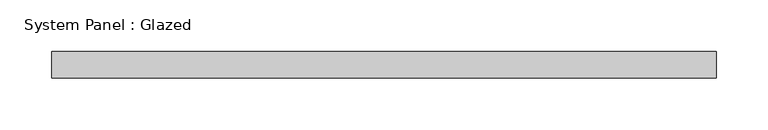
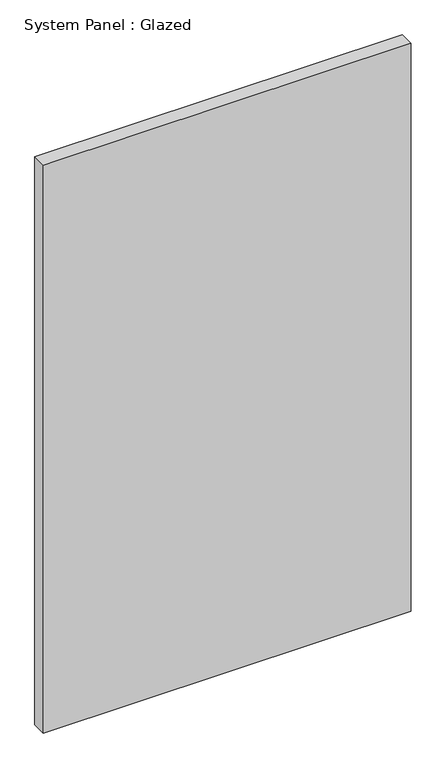
"""IFC4 building model written with IfcOpenShell, lengths in millimetres: plate geometry, System Panel : Glazed."""

from ifc_helpers import new_model, si_unit, origin, origin_with_axes, place, context, project, spatial, polyline, outline, extrude, source, transform, mapped, element, save


def system_panel_glazed_f0f913a6(model_context):
    return source(origin(), model_context, "Body", "SweptSolid", [
        extrude(outline(polyline([(320.675, 19.05), (-320.675, 19.05), (-320.675, 44.45), (320.675, 44.45), (320.675, 19.05)])), origin_with_axes(), (0.0, 0.0, 1.0), 1047.2243728),
    ])


if __name__ == "__main__":
    model = new_model("IFC4")
    model_context = context("Model", 3, world=origin())
    ifc_project = project(units=[si_unit("LENGTHUNIT", "METRE", prefix="MILLI")], contexts=[model_context])
    site = spatial("IfcSite", under=ifc_project)
    building = spatial("IfcBuilding", under=site)
    placement = place(None, origin())
    system_panel_glazed_shape = system_panel_glazed_f0f913a6(model_context)
    element("IfcPlate", 1, ObjectType="System Panel : Glazed", at=placement, inside=building, context=model_context, shape_type="MappedRepresentation", body=[
        mapped(system_panel_glazed_shape, transform((0.0, 0.0, 0.0), x_axis=(1.0, 0.0, 0.0), y_axis=(0.0, 1.0, 0.0), z_axis=(0.0, 0.0, 1.0))),
    ])
    save(model, "model.ifc")

# Revit data of these elements
# Type "System Panel : Glazed"
#   Construction Type Id = "GSP4R"
#   Analytic Construction = "1/8 in Pilkington single glazing"
#   Visual Light Transmittance = 0.9
#   Solar Heat Gain Coefficient = 0.86
#   Heat Transfer Coefficient (U) = 1.18115 BTU/(h·ft²·°F)
#   Define Thermal Properties by = 1
# Element 1 (IfcPlate, "System Panel : Glazed")
#   Materials on its faces: "Glass"
# Materials
#   "Glass": class "Glass", colour RGB 0 128 192, transparency 0.75, Description = "Soda Lime Glass", Cost = 0
